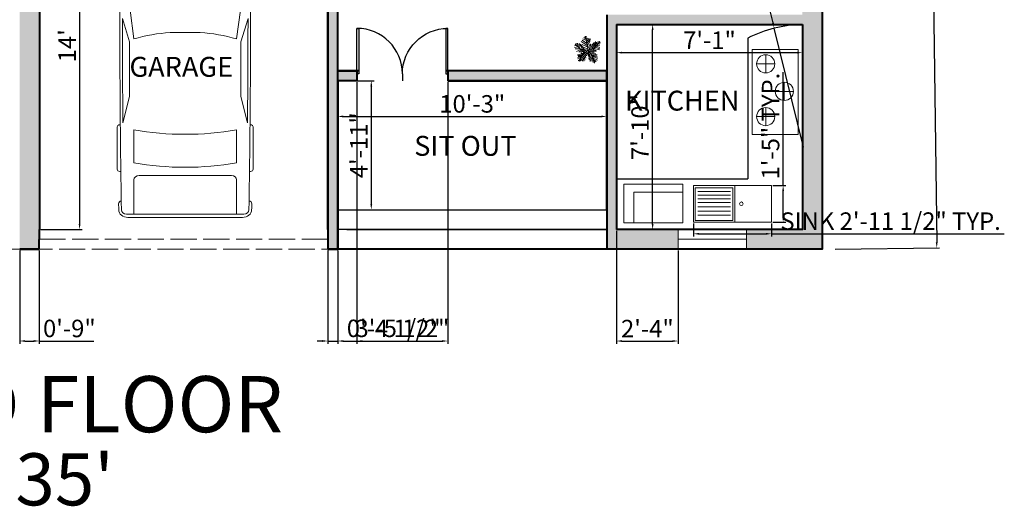
# Model space of a CAD drawing. Units: inches. Extents: x 529 to 1442, y 1029 to 1677.
# Tile 4 of 7: x 991 to 1442, y 1029 to 1252. Entities that reach past the tile are written whole.
import ezdxf

# ---------------------------------------------------------------- set-up
doc = ezdxf.new("R2010")
doc.units = ezdxf.units.IN
doc.linetypes.add('ACAD_ISO02W100', pattern=[15, 12, -3])
for name, color, linetype, lineweight in [('A-ANNO-DIMS', 2, 'Continuous', 18), ('A-ANNO-TEXT', 7, 'Continuous', 30), ('A-AREA-IDEN', 7, 'Continuous', 25), ('A-DOOR', 4, 'Continuous', 25), ('A-EQPM-VEHL', 8, 'Continuous', 13), ('A-FLOR-CASE', 32, 'Continuous', 25), ('A-FLOR-FIXT', 9, 'Continuous', 18), ('A-FLOR-OVHD', 8, 'ACAD_ISO02W100', 18), ('A-FLOR-STRS', 7, 'Continuous', 25), ('A-WALL-PATT', 252, 'Continuous', 13), ('kit', 10, 'Continuous', 18), ('tree', 70, 'Continuous', 13), ('wall', 7, 'Continuous', 40), ('window', 52, 'Continuous', 18)]:
    doc.layers.add(name, color=color, linetype=linetype, lineweight=lineweight)
doc.styles.get("Standard").update_dxf_attribs({"font": 'arial.ttf'})
doc.dimstyles.new('ISO-25', dxfattribs={"dimtxt": 8, "dimasz": 2.5, "dimexe": 1.25, "dimexo": 0.625, "dimtad": 1, "dimdec": 0, "dimlunit": 4, "dimtxsty": 'Standard', "dimcen": 2.5, "dimadec": 0, "dimazin": 0, "dimtfac": 1, "dimtdec": 0, "dimtmove": 0, "dimatfit": 3, "dimfxl": 1, "dimarcsym": 0})

# ---------------------------------------------------------------- blocks, each defined once
blk = doc.blocks.new('*U2')
for p, q in [((0, 0), (0, -6)), ((40, 0), (40, -6))]:
    blk.add_line(p, q)
blk.add_lwpolyline([(0, 0), (0, 40), (1.75, 40), (1.75, 0)], close=True)
blk.add_arc((0, 0), 40, 0, 90)
blk = doc.blocks.new('*U6')
for p, q in [((21.1, 37.41), (21.1, 36.83)), ((46.55, 38.89), (22.35, 38.89)), ((47.8, 37.39), (47.8, 37.41)), ((87.99, 31.87), (74.76, 35.92)), ((134.31, 35.6), (119.29, 31.78)), ((135.45, 37.07), (135.45, 37.41)), ((136.7, 38.89), (160.9, 38.89)), ((162.15, 37.41), (162.15, 36.77)), ((70.03, 31.54), (86.41, 29.35)), ((138.42, 29.35), (157.25, 29.35)), ((186.47, 29.35), (167.01, 29.35)), ((186.47, -33.5), (186.47, 33.5)), ((188.4, -32.76), (188.4, 32.76)), ((164.52, 26.39), (164.52, -26.39)), ((32.27, 11.63), (36.13, 17.17)), ((36.13, 17.17), (50.94, 17.17)), ((3.27, 6.13), (0.1, 0.41)), ((29.77, 9.51), (51.68, 9.51)), ((32.12, 9.51), (32.12, 11.15)), ((58.92, -10.77), (58.92, 10.77)), ((66.55, -10.53), (66.55, 10.53)), ((82.74, 8.5), (82.74, -8.5)), ((186.47, -10.53), (186.47, 10.53)), ((0, 0), (51.68, 0)), ((0.1, -0.41), (3.27, -6.13)), ((29.77, -9.51), (51.68, -9.51)), ((32.12, -9.51), (32.12, -11.15)), ((32.27, -11.63), (36.13, -17.17)), ((36.13, -17.17), (50.94, -17.17)), ((86.41, -29.35), (70.03, -31.54)), ((87.99, -31.87), (74.76, -35.92)), ((134.31, -35.6), (119.29, -31.78)), ((157.25, -29.35), (138.42, -29.35)), ((167.01, -29.35), (186.47, -29.35)), ((21.1, -37.41), (21.1, -36.83)), ((46.55, -38.89), (22.35, -38.89)), ((47.8, -37.39), (47.8, -37.41)), ((135.45, -37.07), (135.45, -37.41)), ((136.7, -38.89), (160.9, -38.89)), ((162.15, -37.41), (162.15, -36.77))]:
    blk.add_line(p, q)
for centre, major_axis, ratio, start_param, end_param in [((266.03, -27.52), (0, 313.31), 0.842304, 1.367076, 1.39176), ((41.19, -490.86), (0, 528.23), 0.842304, 0.00281, 0.075598), ((22.35, 37.41), (0, -1.48), 0.842304, 3.141593, 4.712389), ((64.48, -10555.62), (0, 10593.03), 0.842304, -0.013397, 0.002797), ((46.55, 37.41), (0, 1.48), 0.842304, -1.570796, 0), ((64.48, -10555.62), (0, -10591.55), 0.842304, 3.133765, 3.140441), ((136.7, 37.41), (0, -1.48), 0.842304, 3.141593, 4.712389), ((160.9, 37.41), (0, 1.48), 0.842304, -1.570796, 0), ((180.63, 35.84), (0, 2.22), 0.842304, -0.013017, 1.249894), ((64.48, -10556.36), (0, 10595.31), 0.842304, -0.013397, -0.013017), ((183.98, 33.5), (0, -2.96), 0.842304, 1.570796, 3.128196), ((183.98, 32.76), (0, -5.25), 0.842304, 1.570796, 3.128196), ((259.18, -27.52), (0, -305.3), 0.842304, 4.528606, 4.561838), ((37.47, -593.96), (0, -623.33), 0.842304, 3.096046, 3.200911), ((134.4, 5.39), (0, -89.78), 0.842304, 4.449482, 4.652344), ((135.29, 5.39), (0, 81.77), 0.842304, 1.245306, 1.50788), ((149.6, 2.8), (0, -79.58), 0.842304, 4.372215, 4.640744), ((95.79, -3666.35), (0, -3698.24), 0.842304, 3.134049, 3.144098), ((17.08, 0), (0, 147.02), 0.842304, 4.511394, 4.913384), ((35.91, 0), (0, 147.02), 0.842304, 4.511394, 4.913384), ((167.01, 26.39), (0, 2.96), 0.842304, 0, 1.570796), ((-204.49, 52.4), (0, -250.96), 0.842304, 1.385369, 1.434372), ((13.04, 17.01), (0, 27.42), 0.842304, 4.435146, 4.718221), ((14.2, 17.01), (0, 27.42), 0.842304, 4.435146, 4.718221), ((50.79, 13.34), (6.34, -0.36), 0.603834, -1.395552, 1.581315), ((32.75, 11.15), (0, 0.74), 0.842304, 0.879714, 1.570796), ((29.77, -46.66), (0, 56.17), 0.842304, 0, 0.590319), ((0.62, 0), (0, -0.74), 0.842304, 4.131459, 5.293319), ((29.77, 46.66), (0, 56.17), 0.842304, 2.551274, 3.141593), ((-204.49, -52.4), (0, 250.96), 0.842304, -1.434372, -1.385369), ((32.75, -11.15), (0, -0.74), 0.842304, 4.712389, 5.403472), ((13.04, -17.01), (0, -27.42), 0.842304, 1.564964, 1.848039), ((14.2, -17.01), (0, -27.42), 0.842304, 1.564964, 1.848039), ((134.4, -5.39), (0, -89.78), 0.842304, -1.510751, -1.307889), ((135.29, -5.39), (0, -81.77), 0.842304, -1.50788, -1.245306), ((149.6, -2.8), (0, -79.58), 0.842304, -1.499151, -1.230623), ((259.18, 27.52), (0, 305.3), 0.842304, 1.721348, 1.754579), ((167.01, -26.39), (0, -2.96), 0.842304, 4.712389, 6.283185), ((266.03, 27.52), (0, 313.31), 0.842304, 1.749832, 1.774517), ((37.47, 593.96), (0, -623.33), 0.842304, -0.059319, 0.045547), ((95.79, 3666.35), (0, -3698.24), 0.842304, -0.002505, 0.007544), ((183.98, -33.5), (0, 2.96), 0.842304, 3.15499, 4.712389), ((183.98, -32.76), (0, -5.25), 0.842304, 0.013397, 1.570796), ((41.19, 490.86), (0, -528.23), 0.842304, -0.075598, -0.00281), ((22.35, -37.41), (0, 1.48), 0.842304, 1.570796, 3.141593), ((64.48, 10555.62), (0, 10593.03), 0.842304, 3.138796, 3.15499), ((46.55, -37.41), (0, -1.48), 0.842304, 0, 1.570796), ((64.48, 10555.62), (0, -10591.55), 0.842304, 0.001152, 0.007828), ((136.7, -37.41), (0, -1.48), 0.842304, -1.570796, 0), ((160.9, -37.41), (0, 1.48), 0.842304, 3.141593, 4.712389), ((180.63, -35.84), (0, -2.22), 0.842304, -1.249894, 0.013017), ((64.48, 10556.36), (0, 10595.31), 0.842304, 3.15461, 3.15499)]:
    blk.add_ellipse(centre, major_axis=major_axis, ratio=ratio, start_param=start_param, end_param=end_param)
at = {"extrusion": (0, 0, -1)}
blk.add_ellipse((50.79, -13.34), major_axis=(6.34, 0.36), ratio=0.603834, start_param=-1.395552, end_param=1.581315, dxfattribs=at)
blk = doc.blocks.new('*U12')
for p, q in [((-5.114, 28.097), (-24.676, 40.636)), ((-7.288, 39.707), (-21.778, 46.673)), ((-8.737, 47.138), (-17.069, 52.711)), ((-10.186, 53.64), (-13.084, 55.962)), ((0, 0), (-10.5, 57)), ((-9.099, 51.782), (-6.563, 55.962)), ((-7.65, 43.423), (-2.578, 49.46)), ((-5.839, 35.992), (4.667, 48.067)), ((-5.114, 27.632), (10.463, 46.673)), ((-47.498, 19.737), (-55.83, 18.344)), ((-40.615, 13.7), (-55.105, 10.913)), ((-31.5, 4.5), (-52.5, 25.5)), ((-33.37, 6.269), (-52.207, 5.34)), ((-48.585, 21.131), (-49.309, 29.026)), ((-28.299, 3.483), (-47.86, -5.805)), ((-43.513, 28.561), (-42.427, 15.558)), ((-38.442, 26.239), (-34.819, 7.663)), ((-21.416, 3.018), (-38.079, -8.128)), ((-35.544, 28.097), (-24.314, 3.947)), ((0, 0), (-31.5, 4.5)), ((-14.533, 2.09), (-30.834, 25.31)), ((-15.982, 2.09), (-30.11, -9.521)), ((-3.665, 19.273), (-27.574, 35.527)), ((-24.314, 23.917), (-2.941, 13.7)), ((0, 0), (-22.5, -19.5)), ((-6.563, 1.161), (-21.416, -8.128)), ((-20.691, 13.7), (-1.129, 4.876)), ((-2.941, 16.486), (8.652, 37.85)), ((-1.129, 6.734), (9.014, 26.704)), ((0, 0), (27, 9)), ((0, 0), (18, -22.5)), ((3.942, 1.625), (11.187, 24.381)), ((6.478, 1.625), (26.04, -8.592)), ((10.101, 3.483), (17.708, 26.239)), ((11.187, 3.483), (30.749, -5.805)), ((16.259, 5.805), (23.142, 31.348)), ((18.07, 5.805), (35.096, -3.483)), ((22.055, 7.198), (27.489, 32.277)), ((24.229, 7.663), (46.688, 1.625)), ((27, 9), (48, 36)), ((27.127, 9.056), (31.112, 35.992)), ((29.662, 12.307), (48.137, 6.269)), ((31.836, 30.883), (32.561, 16.486)), ((33.285, 16.486), (48.862, 10.913)), ((35.096, 32.741), (37.27, 22.524)), ((36.183, 19.737), (48.137, 17.88)), ((38.719, 34.134), (41.979, 28.561)), ((40.53, 25.775), (48.862, 24.846)), ((43.791, 29.954), (51.036, 30.883)), ((44.153, 36.456), (45.239, 32.741)), ((-17.431, -15.094), (-42.789, -18.809)), ((-28.299, -29.026), (-42.789, -31.348)), ((-24.314, -21.596), (-42.427, -22.06)), ((-30.834, -34.135), (-42.427, -35.528)), ((-34.457, -39.708), (-40.978, -42.494)), ((-26.849, -26.24), (-40.253, -25.775)), ((-22.5, -19.5), (-37.5, -45)), ((-32.646, -36.921), (-31.921, -44.352)), ((-15.257, -12.772), (-30.11, -12.772)), ((-29.023, -30.884), (-27.936, -43.887)), ((-25.038, -23.918), (-22.865, -45.281)), ((-20.691, -18.345), (-17.793, -44.352)), ((-6.563, -5.805), (-19.967, -9.985)), ((-17.069, -15.094), (-12.721, -40.172)), ((-13.446, -11.378), (-8.737, -32.741)), ((-9.461, -8.592), (-6.201, -23.453)), ((-4.752, -3.483), (-3.665, -14.629)), ((2.493, -3.019), (-1.491, -20.202)), ((1.769, -2.555), (24.229, -9.521)), ((5.029, -6.27), (2.131, -25.775)), ((9.014, -11.378), (3.58, -35.992)), ((14.085, -16.951), (6.478, -40.172)), ((7.565, -9.056), (32.198, -14.629)), ((18.07, -22.524), (8.289, -45.745)), ((12.274, -15.094), (36.907, -18.809)), ((20.244, -30.419), (15.897, -44.816)), ((16.259, -19.738), (36.183, -22.989)), ((18, -22.5), (27, -52.5)), ((18.433, -22.524), (40.53, -29.026)), ((19.157, -25.311), (38.719, -33.206)), ((22.78, -37.85), (19.519, -48.532)), ((21.331, -32.741), (39.081, -40.636)), ((22.78, -38.314), (34.372, -44.816)), ((24.591, -45.745), (23.142, -50.854)), ((24.591, -43.423), (30.749, -47.603)), ((26.764, -49.925), (28.213, -50.854))]:
    blk.add_line(p, q)
blk = doc.blocks.new('*D29')
at = {"layer": 'A-ANNO-DIMS', "color": 0, "lineweight": -2, "transparency": 16777216}
for p, q in [((1348.76, 1249.47), (1279.64, 1249.47)), ((1280.89, 1158.31), (1280.89, 1246.97)), ((1348.76, 1155.81), (1279.64, 1155.81))]:
    blk.add_line(p, q, dxfattribs=at)
at = {"layer": 'A-ANNO-DIMS', "color": 0, "lineweight": 100, "transparency": 16777216}
for points in [[(1280.47, 1246.97), (1281.31, 1246.97), (1280.89, 1249.47)], [(1280.47, 1158.31), (1281.31, 1158.31), (1280.89, 1155.81)]]:
    blk.add_solid(points, dxfattribs=at)
at = {"layer": 'Defpoints', "color": 0, "lineweight": 100, "transparency": 16777216}
for p in [(1280.89, 1249.47), (1349.38, 1249.47), (1349.38, 1155.81)]:
    blk.add_point(p, dxfattribs=at)
at = {"layer": 'A-ANNO-DIMS', "color": 0, "transparency": 16777216, "insert": (1276.18, 1202.64), "char_height": 8, "attachment_point": 5, "rotation": 90}
blk.add_mtext('7\'-10"', dxfattribs=at)
blk = doc.blocks.new('*D30')
at = {"layer": 'A-ANNO-DIMS', "color": 0, "lineweight": -2, "transparency": 16777216}
for p, q in [((1264.38, 1248.84), (1264.38, 1235.4)), ((1349.38, 1248.84), (1349.38, 1235.4)), ((1266.88, 1236.65), (1346.88, 1236.65))]:
    blk.add_line(p, q, dxfattribs=at)
at = {"layer": 'A-ANNO-DIMS', "color": 0, "lineweight": 100, "transparency": 16777216}
for points in [[(1266.88, 1237.07), (1266.88, 1236.23), (1264.38, 1236.65)], [(1346.88, 1237.07), (1346.88, 1236.23), (1349.38, 1236.65)]]:
    blk.add_solid(points, dxfattribs=at)
at = {"layer": 'Defpoints', "color": 0, "lineweight": 100, "transparency": 16777216}
for p in [(1264.38, 1249.47), (1349.38, 1249.47), (1349.38, 1236.65)]:
    blk.add_point(p, dxfattribs=at)
at = {"layer": 'A-ANNO-DIMS', "color": 0, "transparency": 16777216, "insert": (1306.88, 1241.29), "char_height": 8, "attachment_point": 5}
blk.add_mtext('7\'-1"', dxfattribs=at)
blk = doc.blocks.new('*D31')
at = {"layer": 'A-ANNO-DIMS', "color": 0, "lineweight": -2, "transparency": 16777216}
for p, q in [((1136.88, 1223.19), (1136.88, 1206.24)), ((1259.88, 1223.19), (1259.88, 1206.24)), ((1139.38, 1207.49), (1257.38, 1207.49))]:
    blk.add_line(p, q, dxfattribs=at)
at = {"layer": 'A-ANNO-DIMS', "color": 0, "lineweight": 100, "transparency": 16777216}
for points in [[(1139.38, 1207.91), (1139.38, 1207.07), (1136.88, 1207.49)], [(1257.38, 1207.91), (1257.38, 1207.07), (1259.88, 1207.49)]]:
    blk.add_solid(points, dxfattribs=at)
at = {"layer": 'Defpoints', "color": 0, "lineweight": 100, "transparency": 16777216}
for p in [(1136.88, 1223.81), (1259.88, 1223.81), (1259.88, 1207.49)]:
    blk.add_point(p, dxfattribs=at)
at = {"layer": 'A-ANNO-DIMS', "color": 0, "transparency": 16777216, "insert": (1198.38, 1212.2), "char_height": 8, "attachment_point": 5}
blk.add_mtext('10\'-3"', dxfattribs=at)
blk = doc.blocks.new('*D32')
at = {"layer": 'A-ANNO-DIMS', "color": 0, "lineweight": -2, "transparency": 16777216}
for p, q in [((1137.51, 1223.81), (1153.45, 1223.81)), ((1152.2, 1221.31), (1152.2, 1167.31)), ((1137.51, 1164.81), (1153.45, 1164.81))]:
    blk.add_line(p, q, dxfattribs=at)
at = {"layer": 'A-ANNO-DIMS', "color": 0, "lineweight": 100, "transparency": 16777216}
for points in [[(1151.79, 1221.31), (1152.62, 1221.31), (1152.2, 1223.81)], [(1151.79, 1167.31), (1152.62, 1167.31), (1152.2, 1164.81)]]:
    blk.add_solid(points, dxfattribs=at)
at = {"layer": 'Defpoints', "color": 0, "lineweight": 100, "transparency": 16777216}
for p in [(1136.88, 1223.81), (1136.88, 1164.81), (1152.2, 1164.81)]:
    blk.add_point(p, dxfattribs=at)
at = {"layer": 'A-ANNO-DIMS', "color": 0, "transparency": 16777216, "insert": (1147.56, 1194.31), "char_height": 8, "attachment_point": 5, "rotation": 90}
blk.add_mtext('4\'-11"', dxfattribs=at)
blk = doc.blocks.new('*D34')
at = {"layer": 'A-ANNO-DIMS', "color": 0, "lineweight": -2, "transparency": 16777216}
for p, q in [((1001.01, 1323.81), (1020.03, 1323.81)), ((1018.78, 1321.31), (1018.78, 1158.31)), ((1001.01, 1155.81), (1020.03, 1155.81))]:
    blk.add_line(p, q, dxfattribs=at)
at = {"layer": 'A-ANNO-DIMS', "color": 0, "lineweight": 100, "transparency": 16777216}
for points in [[(1018.36, 1321.31), (1019.19, 1321.31), (1018.78, 1323.81)], [(1018.36, 1158.31), (1019.19, 1158.31), (1018.78, 1155.81)]]:
    blk.add_solid(points, dxfattribs=at)
at = {"layer": 'Defpoints', "color": 0, "lineweight": 100, "transparency": 16777216}
for p in [(1000.38, 1323.81), (1000.38, 1155.81), (1018.78, 1155.81)]:
    blk.add_point(p, dxfattribs=at)
at = {"layer": 'A-ANNO-DIMS', "color": 0, "transparency": 16777216, "insert": (1014.13, 1239.81), "char_height": 8, "attachment_point": 5, "rotation": 90}
blk.add_mtext("14'", dxfattribs=at)
blk = doc.blocks.new('*D56')
at = {"layer": 'A-ANNO-DIMS', "color": 0, "lineweight": -2, "transparency": 16777216}
for p, q in [((1359.01, 1566.82), (1406.77, 1567.43)), ((1405.56, 1564.91), (1410.83, 1149.91)), ((1364.34, 1146.82), (1412.11, 1147.43))]:
    blk.add_line(p, q, dxfattribs=at)
at = {"layer": 'A-ANNO-DIMS', "color": 0, "lineweight": 100, "transparency": 16777216}
for points in [[(1405.97, 1564.92), (1405.14, 1564.91), (1405.52, 1567.41)], [(1411.24, 1149.92), (1410.41, 1149.91), (1410.86, 1147.41)]]:
    blk.add_solid(points, dxfattribs=at)
at = {"layer": 'Defpoints', "color": 0, "lineweight": 100, "transparency": 16777216}
for p in [(1358.38, 1566.81), (1363.72, 1146.81), (1410.86, 1147.41)]:
    blk.add_point(p, dxfattribs=at)
at = {"layer": 'A-ANNO-DIMS', "color": 0, "transparency": 16777216, "insert": (1412.9, 1357.47), "char_height": 8, "attachment_point": 5, "rotation": 270.7276}
blk.add_mtext("35'", dxfattribs=at)
blk = doc.blocks.new('WIN-SMALL-PLAN')
blk.add_line((0, 4.5), (31.29, 4.5))
blk.add_lwpolyline([(0, 9), (31.29, 9), (31.29, 0), (0, 0)], close=True)
blk = doc.blocks.new('KITCHEN-COUNTER-UNIT')
for p, q in [((4.66, 0), (4.66, 13.96)), ((4.66, 13.96), (26.96, 13.96))]:
    blk.add_line(p, q)
blk.add_lwpolyline([(0, 17.63), (26.96, 17.63), (26.96, 0), (0, 0)], close=True)
blk = doc.blocks.new('SINK-WITH-DRAINBOARD')
for p, q in [((1.96, 14.02), (16.96, 14.02)), ((18.91, 0), (18.91, 16.76)), ((1.96, 12.32), (16.96, 12.32)), ((1.96, 10.57), (16.96, 10.57)), ((1.96, 8.97), (16.96, 8.97)), ((1.96, 7.02), (16.96, 7.02)), ((1.96, 5.06), (16.96, 5.06)), ((1.96, 3.1), (16.96, 3.1))]:
    blk.add_line(p, q)
for points in [[(0, 0), (35.68, 0), (35.68, 16.76), (0, 16.76)], [(0.77, 15.62), (18.04, 15.62), (18.04, 0.78), (0.77, 0.78)]]:
    blk.add_lwpolyline(points, close=True)
blk.add_circle((21.95, 8.38), 0.822)
blk = doc.blocks.new('COOKTOP-THREE-BURNER')
for p, q in [((6.23, 28.11), (6.23, 36.44)), ((6.23, 36.44), (6.23, 32.27)), ((10.39, 32.27), (2.07, 32.27)), ((6.23, 32.27), (10.39, 32.27)), ((14.71, 15.52), (14.71, 23.85)), ((14.71, 23.85), (14.71, 19.68)), ((18.87, 19.68), (10.54, 19.68)), ((14.71, 19.68), (18.87, 19.68)), ((6.23, 3.99), (6.23, 12.32)), ((6.23, 12.32), (6.23, 8.16)), ((10.39, 8.16), (2.07, 8.16)), ((6.23, 8.16), (10.39, 8.16))]:
    blk.add_line(p, q)
blk.add_lwpolyline([(0, 38.87), (20.99, 38.87), (20.99, 0), (0, 0)], close=True)
for centre in [(6.23, 32.27), (14.71, 19.68), (6.23, 8.16)]:
    blk.add_circle(centre, 4.16)
blk = doc.blocks.new('*D95')
at = {"layer": 'A-ANNO-DIMS', "color": 0, "lineweight": -2, "transparency": 16777216}
for p, q in [((1299.54, 1158.55), (1299.54, 1152.58)), ((1335.22, 1158.55), (1335.22, 1152.58)), ((1302.04, 1153.83), (1332.72, 1153.83)), ((1335.22, 1153.83), (1441.75, 1153.83))]:
    blk.add_line(p, q, dxfattribs=at)
at = {"layer": 'A-ANNO-DIMS', "color": 0, "lineweight": 100, "transparency": 16777216}
for points in [[(1302.04, 1154.24), (1302.04, 1153.41), (1299.54, 1153.83)], [(1332.72, 1154.24), (1332.72, 1153.41), (1335.22, 1153.83)]]:
    blk.add_solid(points, dxfattribs=at)
at = {"layer": 'Defpoints', "color": 0, "lineweight": 100, "transparency": 16777216}
for p in [(1299.54, 1159.18), (1335.22, 1159.18), (1335.22, 1153.83)]:
    blk.add_point(p, dxfattribs=at)
at = {"layer": 'A-ANNO-DIMS', "color": 0, "transparency": 16777216, "insert": (1389.73, 1158.59), "char_height": 8, "attachment_point": 5}
blk.add_mtext('SINK 2\'-11 1/2" TYP.', dxfattribs=at)
blk = doc.blocks.new('*D96')
at = {"layer": 'A-ANNO-DIMS', "color": 0, "lineweight": -2, "transparency": 16777216}
for p, q in [((1340.58, 1175.93), (1340.58, 1227.7)), ((1335.85, 1175.93), (1341.83, 1175.93)), ((1340.58, 1161.68), (1340.58, 1173.43)), ((1335.85, 1159.18), (1341.83, 1159.18))]:
    blk.add_line(p, q, dxfattribs=at)
at = {"layer": 'A-ANNO-DIMS', "color": 0, "lineweight": 100, "transparency": 16777216}
for points in [[(1340.16, 1173.43), (1340.99, 1173.43), (1340.58, 1175.93)], [(1340.16, 1161.68), (1340.99, 1161.68), (1340.58, 1159.18)]]:
    blk.add_solid(points, dxfattribs=at)
at = {"layer": 'Defpoints', "color": 0, "lineweight": 100, "transparency": 16777216}
for p in [(1335.22, 1175.93), (1340.58, 1175.93), (1335.22, 1159.18)]:
    blk.add_point(p, dxfattribs=at)
at = {"layer": 'A-ANNO-DIMS', "color": 0, "transparency": 16777216, "insert": (1335.87, 1203.07), "char_height": 8, "attachment_point": 5, "rotation": 90}
blk.add_mtext('1\'-5" TYP.', dxfattribs=at)
blk = doc.blocks.new('*D112')
at = {"layer": 'A-ANNO-DIMS', "color": 0, "lineweight": -2, "transparency": 16777216}
for p, q in [((1264.38, 1155.19), (1264.38, 1103.56)), ((1292.57, 1146.19), (1292.57, 1103.56)), ((1266.88, 1104.81), (1290.07, 1104.81))]:
    blk.add_line(p, q, dxfattribs=at)
at = {"layer": 'A-ANNO-DIMS', "color": 0, "lineweight": 100, "transparency": 16777216}
for points in [[(1266.88, 1105.23), (1266.88, 1104.4), (1264.38, 1104.81)], [(1290.07, 1105.23), (1290.07, 1104.4), (1292.57, 1104.81)]]:
    blk.add_solid(points, dxfattribs=at)
at = {"layer": 'Defpoints', "color": 0, "lineweight": 100, "transparency": 16777216}
for p in [(1264.38, 1155.81), (1292.57, 1146.81), (1292.57, 1104.81)]:
    blk.add_point(p, dxfattribs=at)
at = {"layer": 'A-ANNO-DIMS', "color": 0, "transparency": 16777216, "insert": (1278.48, 1109.45), "char_height": 8, "attachment_point": 5}
blk.add_mtext('2\'-4"', dxfattribs=at)
blk = doc.blocks.new('*D113')
at = {"layer": 'A-ANNO-DIMS', "color": 0, "lineweight": -2, "transparency": 16777216}
for p, q in [((991.38, 1146.19), (991.38, 1103.56)), ((1000.35, 1146.19), (1000.35, 1103.56)), ((993.88, 1104.81), (997.85, 1104.81)), ((1000.35, 1104.81), (1025.36, 1104.81))]:
    blk.add_line(p, q, dxfattribs=at)
at = {"layer": 'A-ANNO-DIMS', "color": 0, "lineweight": 100, "transparency": 16777216}
for points in [[(993.88, 1105.23), (993.88, 1104.4), (991.38, 1104.81)], [(997.85, 1105.23), (997.85, 1104.4), (1000.35, 1104.81)]]:
    blk.add_solid(points, dxfattribs=at)
at = {"layer": 'Defpoints', "color": 0, "lineweight": 100, "transparency": 16777216}
for p in [(991.38, 1146.81), (1000.35, 1146.81), (1000.35, 1104.81)]:
    blk.add_point(p, dxfattribs=at)
at = {"layer": 'A-ANNO-DIMS', "color": 0, "transparency": 16777216, "insert": (1014.1, 1109.52), "char_height": 8, "attachment_point": 5}
blk.add_mtext('0\'-9"', dxfattribs=at)
blk = doc.blocks.new('*D114')
at = {"layer": 'A-ANNO-DIMS', "color": 0, "lineweight": -2, "transparency": 16777216}
for p, q in [((1132.38, 1146.19), (1132.38, 1103.56)), ((1136.88, 1146.19), (1136.88, 1103.56)), ((1129.88, 1104.81), (1127.38, 1104.81)), ((1132.38, 1104.81), (1136.88, 1104.81)), ((1139.38, 1104.81), (1183.04, 1104.81))]:
    blk.add_line(p, q, dxfattribs=at)
at = {"layer": 'A-ANNO-DIMS', "color": 0, "lineweight": 100, "transparency": 16777216}
for points in [[(1129.88, 1105.23), (1129.88, 1104.4), (1132.38, 1104.81)], [(1139.38, 1105.23), (1139.38, 1104.4), (1136.88, 1104.81)]]:
    blk.add_solid(points, dxfattribs=at)
at = {"layer": 'Defpoints', "color": 0, "lineweight": 100, "transparency": 16777216}
for p in [(1132.38, 1146.81), (1136.88, 1146.81), (1136.88, 1104.81)]:
    blk.add_point(p, dxfattribs=at)
at = {"layer": 'A-ANNO-DIMS', "color": 0, "transparency": 16777216, "insert": (1162.46, 1109.57), "char_height": 8, "attachment_point": 5}
blk.add_mtext('0\'-4 1/2"', dxfattribs=at)
blk = doc.blocks.new('*D116')
at = {"layer": 'A-ANNO-DIMS', "color": 0, "lineweight": -2, "transparency": 16777216}
for p, q in [((1145.62, 1223.19), (1145.62, 1103.56)), ((1187.26, 1223.19), (1187.26, 1103.56)), ((1148.12, 1104.81), (1184.76, 1104.81))]:
    blk.add_line(p, q, dxfattribs=at)
at = {"layer": 'A-ANNO-DIMS', "color": 0, "lineweight": 100, "transparency": 16777216}
for points in [[(1148.12, 1105.23), (1148.12, 1104.4), (1145.62, 1104.81)], [(1184.76, 1105.23), (1184.76, 1104.4), (1187.26, 1104.81)]]:
    blk.add_solid(points, dxfattribs=at)
at = {"layer": 'Defpoints', "color": 0, "lineweight": 100, "transparency": 16777216}
for p in [(1145.62, 1223.81), (1187.26, 1223.81), (1187.26, 1104.81)]:
    blk.add_point(p, dxfattribs=at)
at = {"layer": 'A-ANNO-DIMS', "color": 0, "transparency": 16777216, "insert": (1166.44, 1109.58), "char_height": 8, "attachment_point": 5}
blk.add_mtext('3\'-5 1/2"', dxfattribs=at)
blk = doc.blocks.new('*D117')
at = {"layer": 'A-ANNO-DIMS', "color": 0, "lineweight": -2, "transparency": 16777216}
for p, q in [((1324.84, 1295.1), (1335.92, 1250.26)), ((1349.96, 1193.47), (1336.52, 1247.84))]:
    blk.add_line(p, q, dxfattribs=at)
at = {"layer": 'A-ANNO-DIMS', "color": 0, "lineweight": 100, "transparency": 16777216}
blk.add_solid([(1336.33, 1250.36), (1335.52, 1250.16), (1336.52, 1247.84)], dxfattribs=at)
at = {"layer": 'Defpoints', "color": 0, "lineweight": 100, "transparency": 16777216}
for p in [(1336.52, 1247.84), (1349.96, 1193.47)]:
    blk.add_point(p, dxfattribs=at)
at = {"layer": 'A-ANNO-DIMS', "color": 0, "transparency": 16777216, "insert": (1333.03, 1281.58), "char_height": 8, "attachment_point": 5, "rotation": 283.8857}
blk.add_mtext('R4\'-8"', dxfattribs=at)

msp = doc.modelspace()

# ---------------------------------------------------------------- hatches: boundary and pattern name
at = {"layer": 'A-WALL-PATT'}
h = msp.add_hatch(color=256, dxfattribs=at)
h.dxf.hatch_style = 1
h.paths.add_polyline_path([(1031.09, 1566.81), (959.72, 1566.81), (959.72, 1557.81), (991.38, 1557.81), (1031.09, 1557.81)])
h.paths.add_polyline_path([(1000.38, 1557.81), (991.38, 1557.81), (991.38, 1413.81), (991.38, 1409.31), (1000.38, 1409.31)])
h.paths.add_polyline_path([(991.38, 1413.81), (904.07, 1413.81), (904.07, 1409.31), (991.38, 1409.31)])
h.paths.add_polyline_path([(931.38, 1409.31), (926.88, 1409.31), (926.88, 1359.54), (931.38, 1359.54)])
h.paths.add_polyline_path([(854.88, 1257.31), (835.24, 1257.31), (835.24, 1252.81), (854.36, 1252.81, -0.003534), (854.88, 1252.81)])
h.paths.add_polyline_path([(859.38, 1323.81), (991.38, 1323.81), (991.38, 1328.31), (931.38, 1328.31), (854.88, 1328.31), (854.88, 1155.81), (859.38, 1155.81)])
h.paths.add_polyline_path([(1000.38, 1323.81), (991.38, 1323.81), (991.38, 1155.81), (991.38, 1146.81), (1000.35, 1146.81), (1000.38, 1155.81)])
h.paths.add_polyline_path([(1041.38, 1328.31), (1000.38, 1328.31), (1000.38, 1323.81), (1041.38, 1323.81)])
h.paths.add_polyline_path([(1041.38, 1339.12), (1036.88, 1339.12), (1036.88, 1328.31), (1041.38, 1328.31)])
h.paths.add_polyline_path([(1000.38, 1328.31), (991.38, 1328.31), (991.38, 1323.81), (1000.38, 1323.81)])
h.paths.add_polyline_path([(1041.38, 1409.31), (1036.88, 1409.31), (1036.88, 1360.41), (1041.38, 1360.41)])
h.paths.add_polyline_path([(1042.64, 1413.81), (1000.38, 1413.81), (1000.38, 1409.31), (1042.64, 1409.31)])
h = msp.add_hatch(color=256, dxfattribs=at)
h.dxf.hatch_style = 1
h.paths.add_polyline_path([(1160.38, 1566.81), (1099.95, 1566.81), (1099.95, 1557.81), (1132.38, 1557.81), (1160.38, 1557.81)])
h.paths.add_polyline_path([(1136.88, 1557.81), (1132.38, 1557.81), (1132.38, 1457.46), (1136.88, 1457.46)])
h.paths.add_polyline_path([(1171.8, 1467.81), (1136.88, 1467.81), (1136.88, 1463.31), (1171.8, 1463.31)])
h.paths.add_polyline_path([(1212.38, 1557.81), (1207.88, 1557.81), (1207.88, 1467.81), (1207.88, 1409.31), (1218.04, 1409.31), (1218.04, 1413.81), (1212.38, 1413.81), (1212.38, 1463.31)])
h.paths.add_polyline_path([(1136.88, 1409.31), (1132.38, 1409.31), (1132.38, 1146.81), (1136.88, 1146.81)])
h.paths.add_polyline_path([(1136.88, 1417.46), (1132.38, 1417.46), (1132.38, 1409.31), (1136.88, 1409.31)])
h.paths.add_polyline_path([(1132.38, 1413.81), (1075.12, 1413.81), (1075.12, 1409.31), (1132.38, 1409.31)])
h.paths.add_polyline_path([(1132.38, 1328.31), (1041.38, 1328.31), (1041.38, 1323.81), (1132.38, 1323.81)])
h = msp.add_hatch(color=256, dxfattribs=at)
h.dxf.hatch_style = 1
h.paths.add_polyline_path([(1259.88, 1228.31), (1187.26, 1228.31), (1187.26, 1226.94), (1187.26, 1223.81), (1259.88, 1223.81)])
h.paths.add_polyline_path([(1145.62, 1226.94), (1145.62, 1228.31), (1136.88, 1228.31), (1136.88, 1223.81), (1145.62, 1223.81)])
h.paths.add_polyline_path([(1136.88, 1228.31), (1132.38, 1228.31), (1132.38, 1146.81), (1136.88, 1146.81)])
h.paths.add_polyline_path([(1136.88, 1417.46), (1132.38, 1417.46), (1132.38, 1228.31), (1136.88, 1228.31)])
h = msp.add_hatch(color=256, dxfattribs=at)
h.dxf.hatch_style = 1
h.paths.add_polyline_path([(1292.57, 1155.81), (1264.38, 1155.81), (1264.38, 1146.81), (1292.57, 1146.81)], flags=17)
h.paths.add_polyline_path([(1358.38, 1269.29), (1349.38, 1269.29), (1349.38, 1259.81), (1349.38, 1155.81), (1323.86, 1155.81), (1323.86, 1146.81), (1358.38, 1146.81)])
h.paths.add_polyline_path([(1264.38, 1249.47), (1349.38, 1249.47), (1349.38, 1253.97), (1259.88, 1253.97), (1259.88, 1164.81), (1259.88, 1146.81), (1264.38, 1146.81), (1264.38, 1155.81)])

# ---------------------------------------------------------------- linework, layer by layer
at = {"layer": 'A-FLOR-CASE'}
for p in [(1324.38, 1243.29), (1264.38, 1178.98)]:
    msp.add_line(p, (1324.38, 1178.98), dxfattribs=at)
msp.add_arc((1349.96, 1193.47), 56, 90.5931, 117.1782, dxfattribs=at)
at = {"layer": 'A-FLOR-OVHD'}
for p, q in [((1140.88, 1164.81), (1136.88, 1164.81)), ((1136.88, 1164.81), (1259.88, 1164.81)), ((1000.36, 1151.31), (1132.38, 1151.31)), ((859.38, 1146.81), (1132.38, 1146.81))]:
    msp.add_line(p, q, dxfattribs=at)
at = {"layer": 'A-FLOR-STRS'}
for p, q in [((1140.88, 1164.81), (1259.88, 1164.81)), ((1141.06, 1155.81), (1260.06, 1155.81))]:
    msp.add_line(p, q, dxfattribs=at)
msp.add_lwpolyline([(1259.88, 1155.81), (1136.88, 1155.81)], dxfattribs=at)
at = {"layer": 'wall'}
for p, q in [((1358.38, 1566.81), (1358.38, 1146.81)), ((1136.88, 1164.81), (1136.88, 1328.31)), ((1000.38, 1323.81), (1000.38, 1155.81)), ((1132.38, 1155.81), (1132.38, 1323.81)), ((1259.88, 1253.97), (1259.88, 1164.81)), ((1264.38, 1249.47), (1264.38, 1155.81)), ((1264.38, 1249.47), (1349.38, 1249.47)), ((1132.38, 1228.31), (1132.38, 1155.81)), ((1146.53, 1228.31), (1136.88, 1228.31)), ((1166.49, 1228.31), (1166.4, 1228.31)), ((1259.88, 1228.31), (1186.35, 1228.31)), ((1136.88, 1223.81), (1136.88, 1164.81)), ((1145.62, 1223.81), (1136.88, 1223.81)), ((1259.88, 1223.81), (1187.26, 1223.81)), ((1259.88, 1164.81), (1259.88, 1223.81)), ((1136.88, 1184.96), (1136.88, 1164.81)), ((1136.88, 1164.81), (1136.88, 1146.81)), ((1259.88, 1164.81), (1259.88, 1146.81)), ((1000.35, 1146.81), (1000.38, 1155.81)), ((1132.38, 1155.81), (1132.38, 1146.81)), ((991.38, 1146.81), (1000.35, 1146.81)), ((1000.35, 1146.81), (991.38, 1146.81)), ((1358.38, 1146.81), (1132.38, 1146.81))]:
    msp.add_line(p, q, dxfattribs=at)
for points in [[(859.38, 1146.81), (638.38, 1146.81), (638.38, 1566.81), (1358.38, 1566.81), (1358.38, 1146.81), (1132.38, 1146.81)], [(1349.38, 1249.47), (1349.38, 1155.81), (1264.38, 1155.81)], [(1000.35, 1146.81), (991.38, 1146.81)]]:
    msp.add_lwpolyline(points, dxfattribs=at)
for points in [[(1132.38, 1146.81), (1136.88, 1146.81), (1136.88, 1417.46), (1132.38, 1417.46)], [(1145.62, 1223.81), (1136.88, 1223.81), (1136.88, 1228.31), (1145.62, 1228.31)], [(1187.26, 1223.81), (1259.88, 1223.81), (1259.88, 1228.31), (1187.26, 1228.31)]]:
    msp.add_lwpolyline(points, close=True, dxfattribs=at)

# ---------------------------------------------------------------- block references
at = {"layer": 'A-DOOR', "yscale": 0.5205824161454354, "zscale": 0.5205824161454354}
for p, xscale in [((1145.62, 1226.94), 0.5205824161454354), ((1187.26, 1226.94), -0.5205824161454354)]:
    msp.add_blockref('*U2', p, dxfattribs=dict(at, xscale=xscale))
at = {"layer": 'A-EQPM-VEHL', "xscale": 0.7999897948579066, "yscale": 0.7999897948579066, "zscale": 0.7999897948579066, "rotation": 270}
msp.add_blockref('*U6', (1067.08, 1312.04), dxfattribs=at)
at = {"layer": 'A-FLOR-FIXT'}
msp.add_blockref('SINK-WITH-DRAINBOARD', (1299.54, 1159.18), dxfattribs=at)
at = {"layer": 'kit'}
for name, p in [('COOKTOP-THREE-BURNER', (1326.4, 1199.26)), ('KITCHEN-COUNTER-UNIT', (1267.69, 1158.84))]:
    msp.add_blockref(name, p, dxfattribs=at)
at = {"layer": 'tree', "xscale": 0.1116431773080361, "yscale": 0.1116431773080361, "zscale": 0.1116431773080361}
msp.add_blockref('*U12', (1251.35, 1237.76), dxfattribs=at)
at = {"layer": 'window'}
msp.add_blockref('WIN-SMALL-PLAN', (1292.57, 1146.81), dxfattribs=at)

# ---------------------------------------------------------------- texts
at = {"layer": 'A-ANNO-TEXT', "attachment_point": 1}
for s, width, gutter_width, insert, char_height in [('GROUND FLOOR', 6670.8961, 128.42, (844.27, 1088.78), 25.6842), ("60'*35'", 1883.7147, 119.06, (929.17, 1053.48), 23.811)]:
    msp.add_mtext_dynamic_manual_height_columns(s, width=width, gutter_width=gutter_width, heights=[0], dxfattribs=dict(at, insert=insert, char_height=char_height))
at = {"layer": 'A-AREA-IDEN', "char_height": 9.098, "attachment_point": 1}
for s, insert in [('GARAGE', (1041.6, 1234.73)), ('KITCHEN', (1268.25, 1219.26)), ('SIT OUT', (1171.84, 1198.6))]:
    msp.add_mtext_dynamic_manual_height_columns(s, width=307.5887, gutter_width=45.49, heights=[0], dxfattribs=dict(at, insert=insert))

# ---------------------------------------------------------------- dimensions: what is measured, and where the dimension line sits
at = {"layer": 'A-ANNO-DIMS'}
dim = msp.add_aligned_dim(p1=(1358.38, 1566.81), p2=(1363.72, 1146.81), distance=47.14, dimstyle='ISO-25', override={"dimclrd": 0, "dimclre": 0, "dimclrt": 0}, dxfattribs=at)
dim.commit()
dim.dimension.update_dxf_attribs({"geometry": '*D56', "text_midpoint": (1412.9, 1357.47)})
for base, p1, p2, picture, middle in [((1018.78, 1155.81), (1000.38, 1323.81), (1000.38, 1155.81), '*D34', (1014.13, 1239.81)), ((1280.89, 1249.47), (1349.38, 1155.81), (1349.38, 1249.47), '*D29', (1276.18, 1202.64)), ((1152.2, 1164.81), (1136.88, 1223.81), (1136.88, 1164.81), '*D32', (1147.56, 1194.31))]:
    dim = msp.add_linear_dim(base=base, p1=p1, p2=p2, angle=90, dimstyle='ISO-25', override={"dimclrd": 0, "dimclre": 0, "dimclrt": 0}, dxfattribs=at)
    dim.commit()
    dim.dimension.update_dxf_attribs({"geometry": picture, "text_midpoint": middle})
dim = msp.add_radius_dim(center=(1349.96, 1193.47), mpoint=(1336.52, 1247.84), dimstyle='ISO-25', override={"dimdec": 1, "dimlfac": 1, "dimrnd": 0, "dimzin": 1, "dimdsep": 46, "dimlunit": 4, "dimfrac": 2}, dxfattribs=at)
dim.commit()
dim.dimension.update_dxf_attribs({"geometry": '*D117', "text_midpoint": (1328.46, 1280.45), "dimtype": 164})
for base, p1, p2, override, picture, middle in [((1349.38, 1236.65), (1264.38, 1249.47), (1349.38, 1249.47), {"dimclrd": 0, "dimclre": 0, "dimclrt": 0}, '*D30', (1306.88, 1241.29)), ((1259.88, 1207.49), (1136.88, 1223.81), (1259.88, 1223.81), {"dimclrd": 0, "dimclre": 0, "dimclrt": 0}, '*D31', (1198.38, 1212.2)), ((1187.26, 1104.81), (1145.62, 1223.81), (1187.26, 1223.81), {"dimdec": 1, "dimlfac": 1, "dimrnd": 0, "dimzin": 1, "dimdsep": 46, "dimlunit": 4, "dimfrac": 2}, '*D116', (1166.44, 1109.58)), ((1292.57, 1104.81), (1264.38, 1155.81), (1292.57, 1146.81), {"dimdec": 1, "dimlfac": 1, "dimrnd": 0, "dimzin": 1, "dimdsep": 46, "dimlunit": 4, "dimfrac": 2}, '*D112', (1278.48, 1109.45)), ((1000.35, 1104.81), (991.38, 1146.81), (1000.35, 1146.81), {"dimdec": 1, "dimlfac": 1, "dimrnd": 0, "dimzin": 1, "dimdsep": 46, "dimlunit": 4, "dimfrac": 2}, '*D113', (1014.1, 1109.52)), ((1136.88, 1104.81), (1132.38, 1146.81), (1136.88, 1146.81), {"dimdec": 1, "dimlfac": 1, "dimrnd": 0, "dimzin": 1, "dimdsep": 46, "dimlunit": 4, "dimfrac": 2}, '*D114', (1162.46, 1109.57))]:
    dim = msp.add_linear_dim(base=base, p1=p1, p2=p2, dimstyle='ISO-25', override=override, dxfattribs=at)
    dim.commit()
    dim.dimension.update_dxf_attribs({"geometry": picture, "text_midpoint": middle})
dim = msp.add_linear_dim(base=(1340.5754, 1175.9349), p1=(1335.2235, 1159.1781), p2=(1335.2235, 1175.9349), angle=90, text='<> TYP.', dimstyle='ISO-25', override={"dimdec": 1, "dimlfac": 1, "dimrnd": 0, "dimzin": 1, "dimdsep": 46, "dimlunit": 4, "dimfrac": 2}, dxfattribs=at)
dim.commit()
dim.dimension.update_dxf_attribs({"geometry": '*D96', "text_midpoint": (1335.8659, 1203.0653)})
dim = msp.add_linear_dim(base=(1335.22, 1153.83), p1=(1299.54, 1159.18), p2=(1335.22, 1159.18), text='SINK <> TYP.', dimstyle='ISO-25', override={"dimdec": 1, "dimlfac": 1, "dimrnd": 0, "dimzin": 1, "dimdsep": 46, "dimlunit": 4, "dimfrac": 2}, dxfattribs=at)
dim.commit()
dim.dimension.update_dxf_attribs({"geometry": '*D95', "text_midpoint": (1389.73, 1158.59)})

doc.saveas('drawing.dxf')
